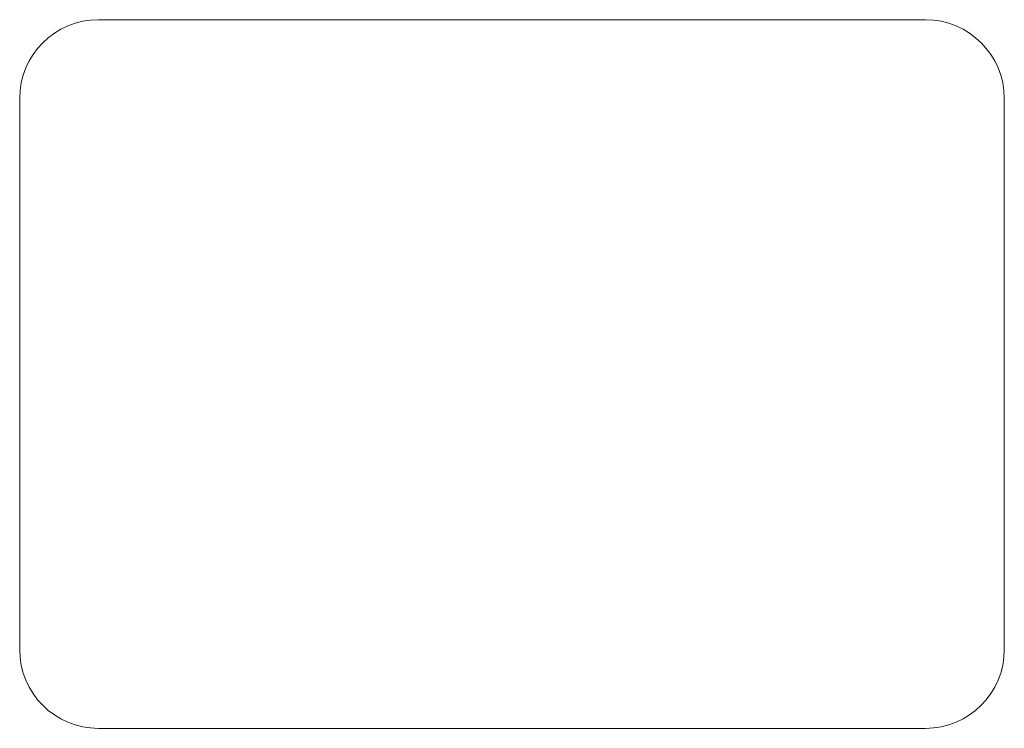
# Model space of a CAD drawing. Units: millimetres. Extents: x 175 to 300, y 109 to 199.
import ezdxf

# ---------------------------------------------------------------- set-up
doc = ezdxf.new("R2010")
doc.units = ezdxf.units.MM
doc.layers.add('M-CONS', color=8, linetype='Continuous', lineweight=18)

msp = doc.modelspace()

# ---------------------------------------------------------------- linework, layer by layer
at = {"layer": 'M-CONS'}
for p, q in [((185.42, 198.57), (290.42, 198.57)), ((175.42, 118.57), (175.42, 188.57)), ((300.42, 188.57), (300.42, 118.57)), ((290.42, 108.57), (185.42, 108.57))]:
    msp.add_line(p, q, dxfattribs=at)
for centre, start, end in [((185.42, 188.57), 90, 180), ((290.42, 188.57), 0, 90), ((185.42, 118.57), 180, 270), ((290.42, 118.57), 270, 0)]:
    msp.add_arc(centre, 10, start, end, dxfattribs=at)

doc.saveas('drawing.dxf')
